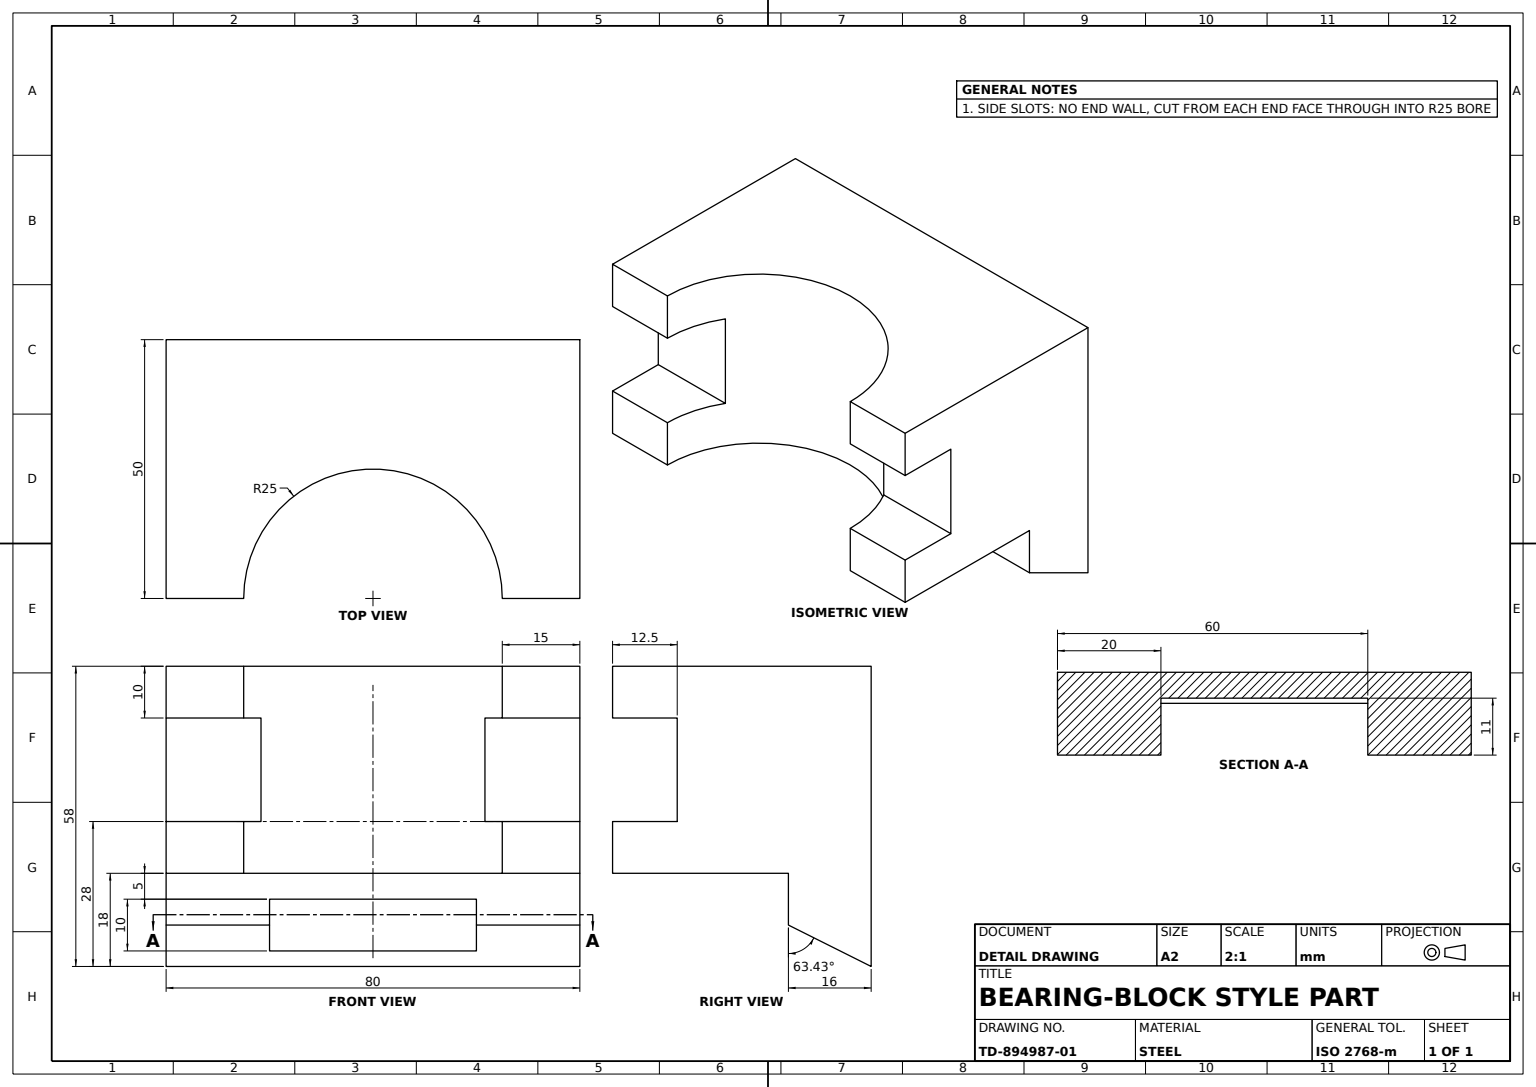
SolidWorks part; units mm, degrees
material "Plain Carbon Steel"
ref_plane "Front Plane" through (0, 0, 0) normal (0, 0, 1) x (1, 0, 0)
ref_plane "Top Plane" through (0, 0, 0) normal (0, 1, 0) x (1, 0, 0)
ref_plane "Right Plane" through (0, 0, 0) normal (1, 0, 0) x (0, 0, -1)
sketch "Base Block Sketch" plane through (0, 0, 0) normal (0, 0, 1) x (1, 0, 0)
  line L0 (0, 0) -> (0, -58)
  line L1 (0, 0) -> (80, 0)
  line L2 (80, 0) -> (80, -58)
  line L3 (80, -58) -> (0, -58)
  dimension "D1" = 80
  dimension "D2" = 58
extrude "Base Block" add sketch "Base Block Sketch" along normal blind 16
sketch "Upper Block Sketch" plane through (0, 0, 0) normal (0, 1, 0) x (1, 0, 0)
  line L0 (0, -16) -> (0, -50)
  line L1 (0, -50) -> (15, -50)
  line L3 (65, -50) -> (80, -50)
  line L4 (80, -50) -> (80, -16)
  line L5 (80, -16) -> (0, -16)
  line L7 (80, 0) -> (0, 0) construction
  arc A0 (65, -50) -> (15, -50) centre (40, -50) ccw
  dimension "D1" = 50
  dimension "D2" = 25
  dimension "D3" = 50
extrude "Upper Block" add sketch "Upper Block Sketch" against normal blind 10
sketch "Side Block Sketch" plane through (0, 0, 0) normal (-1, 0, 0) x (0, 0, 1)
  line L0 (0, 0) -> (0, -58) construction
  line L1 (16, -58) -> (0, -58) construction
  line L2 (25, -10) -> (50, -10) construction
  line L3 (37.5, -10) -> (37.5, -30)
  line L4 (37.5, -30) -> (50, -30)
  line L5 (50, -30) -> (50, -40)
  line L6 (50, -40) -> (16, -40)
  line L7 (16, -10) -> (16, -58) construction
  line L8 (16, -40) -> (16, -10)
  line L9 (16, -10) -> (37.5, -10)
  dimension "D1" = 50
  dimension "D2" = 18
  dimension "D3" = 28
extrude "Side Block 80" add sketch "Side Block Sketch" against normal blind 80
sketch "Bore Ø50 Sketch" plane through (0, -10, 0) normal (0, 1, 0) x (1, 0, 0)
  line L0 (80, -50) -> (0, -50) construction
  line L1 (18.3494, -37.5) -> (61.6506, -37.5)
  line L2 (80, -37.5) -> (0, -37.5) construction
  arc A0 (61.6506, -37.5) -> (18.3494, -37.5) centre (40, -50) ccw
  dimension "D1" = 50
extrude "Semicircular Bore Ø50" cut sketch "Bore Ø50 Sketch" against normal blind 30
sketch "Rectangular Slot Sketch" plane through (0, -40, 0) normal (0, -1, 0) x (1, 0, 0)
  line L0 (18.3494, 37.5) -> (18.3494, 50)
  line L1 (80, 50) -> (0, 50) construction
  line L2 (18.3494, 50) -> (61.6506, 50)
  line L3 (61.6506, 50) -> (61.6506, 37.5)
  line L4 (61.6506, 37.5) -> (18.3494, 37.5)
extrude "Rectangular Slot" cut sketch "Rectangular Slot Sketch" against normal blind 10
sketch "Bore Grooves Sketch" plane through (0, -30, 0) normal (0, 1, 0) x (1, 0, 0)
  line L0 (15, -50) -> (18.3494, -50)
  line L1 (18.3494, -50) -> (18.3494, -37.5)
  line L3 (65, -50) -> (61.6506, -50)
  line L4 (61.6506, -50) -> (61.6506, -37.5)
  line L5 (61.6506, -37.5) -> (61.6506, -50) construction
  arc A0 (65, -50) -> (15, -50) centre (40, -50) ccw construction
  arc A1 (65, -50) -> (61.6506, -37.5) centre (40, -50) ccw
  arc A2 (18.3494, -37.5) -> (15, -50) centre (40, -50) ccw
  dimension "D1" = 50
extrude "Bore Side Grooves" cut sketch "Bore Grooves Sketch" against normal blind 10
sketch "Wedge Cut Sketch" plane through (0, 0, 0) normal (-1, 0, 0) x (0, 0, 1)
  line L0 (16, -40) -> (50, -40) construction
  line L1 (16, -40) -> (16, -58) construction
  line L2 (16, -50) -> (0, -58)
  line L3 (0, 0) -> (0, -58) construction
  line L4 (0, -58) -> (16, -58)
  line L5 (16, -58) -> (16, -50)
  dimension "D1" = 10
extrude "Wedge Cut" cut sketch "Wedge Cut Sketch" against normal blind 80
sketch "Bottom Notch Sketch" plane through (0, 0, 16) normal (0, 0, 1) x (1, 0, 0)
  line L0 (0, -40) -> (0, -50) construction
  line L1 (80, -50) -> (0, -50) construction
  line L2 (60, -50) -> (60, -45)
  line L3 (60, -45) -> (20, -45)
  line L4 (20, -45) -> (20, -55)
  line L5 (20, -55) -> (60, -55)
  line L6 (60, -55) -> (60, -50)
  dimension "D1" = 20
  dimension "D2" = 60
  dimension "D3" = 5
extrude "Bottom Notch" cut sketch "Bottom Notch Sketch" against normal blind 11
